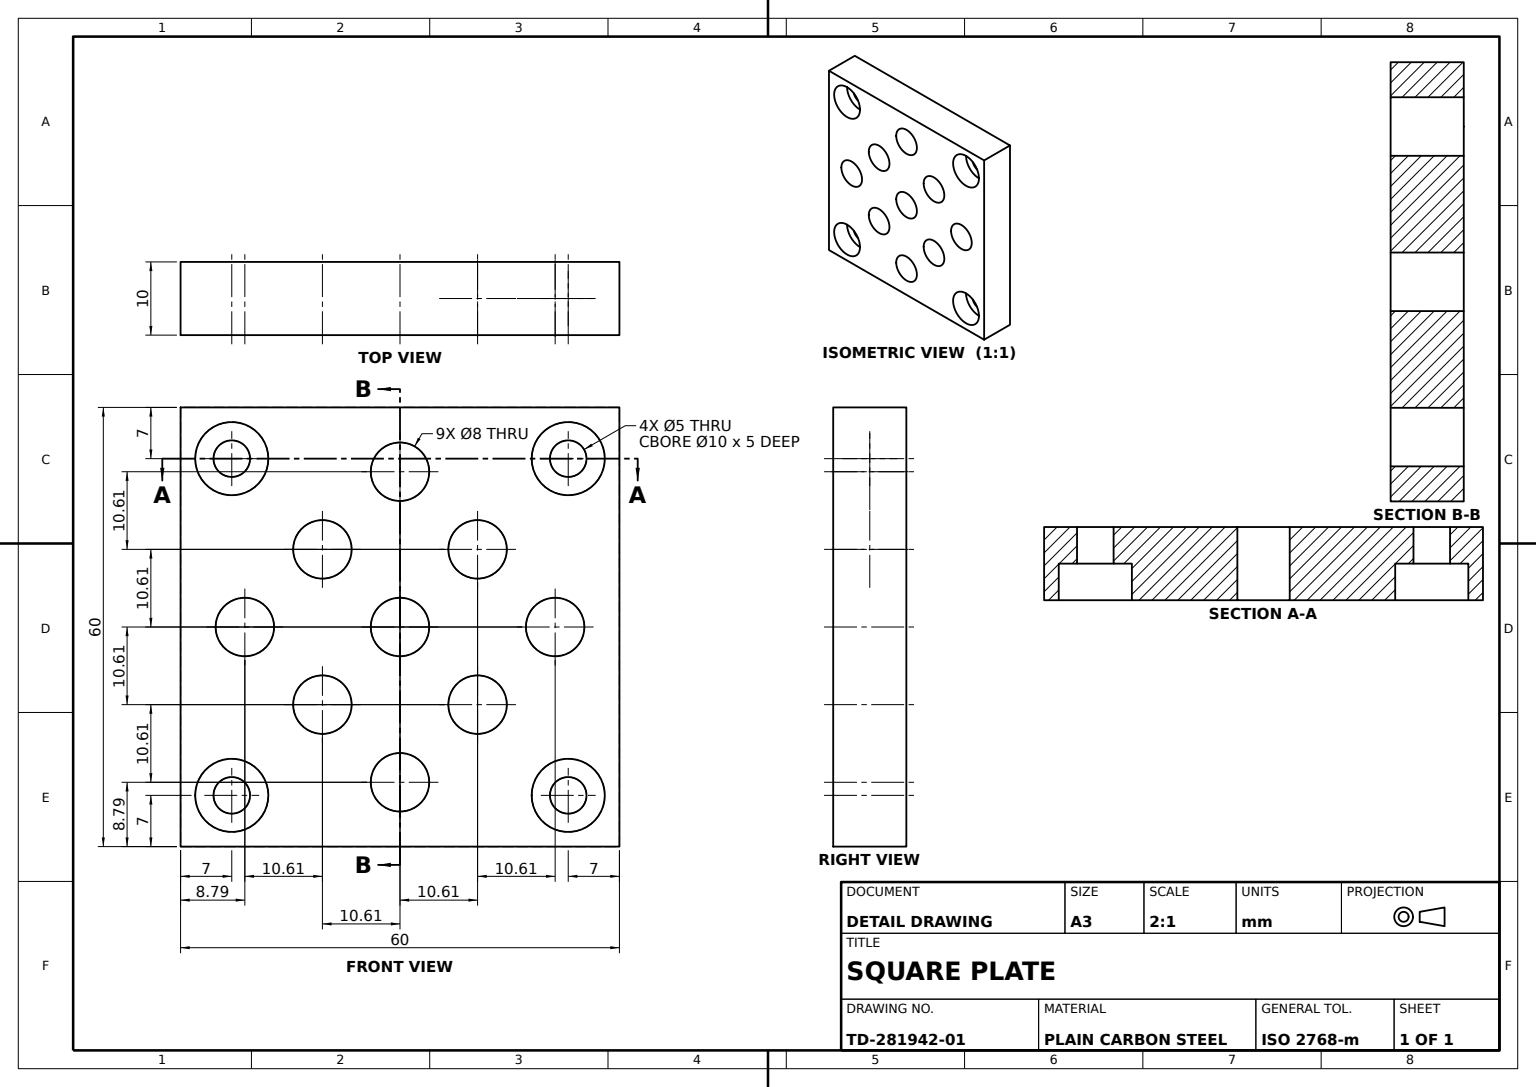
from build123d import *

# Parameters (mm, degrees)
PLATE_PROFILE_60X60_W           = 60
PLATE_PROFILE_60X60_H           = 60
BASE_PLATE_60X60X10_DEPTH       = 10
COUNTERBORE_PROFILE_4X_10_R     = 5
CORNER_COUNTERBORES_4X_10_DEPTH = 5
CORNER_HOLE_PROFILE_4X_5_R      = 2.5
CORNER_HOLES_4X_5_DEPTH         = 5
INNER_THROUGH_HOLES_12X_DEPTH   = 10


with BuildPart() as part:
    # Plate Profile 60x60 → Base Plate 60x60x10 (new body)
    with BuildSketch(Plane.XY):
        with Locations((30, 30)):
            Rectangle(PLATE_PROFILE_60X60_W, PLATE_PROFILE_60X60_H)
    extrude(amount=BASE_PLATE_60X60X10_DEPTH)

    # Counterbore Profile 4xØ10 → Corner Counterbores 4xØ10 (cut)
    with BuildSketch(Plane.XY.offset(10)):
        with Locations((7, 53)):
            Circle(COUNTERBORE_PROFILE_4X_10_R)
        with Locations((53, 53)):
            Circle(COUNTERBORE_PROFILE_4X_10_R)
        with Locations((7, 7)):
            Circle(COUNTERBORE_PROFILE_4X_10_R)
        with Locations((53, 7)):
            Circle(COUNTERBORE_PROFILE_4X_10_R)
    extrude(amount=-CORNER_COUNTERBORES_4X_10_DEPTH, mode=Mode.SUBTRACT)

    # Corner Hole Profile 4xØ5 → Corner Holes 4xØ5 (cut)
    with BuildSketch(Plane.XY.offset(5)):
        with Locations((7, 53)):
            Circle(CORNER_HOLE_PROFILE_4X_5_R)
        with Locations((53, 53)):
            Circle(CORNER_HOLE_PROFILE_4X_5_R)
        with Locations((7, 7)):
            Circle(CORNER_HOLE_PROFILE_4X_5_R)
        with Locations((53, 7)):
            Circle(CORNER_HOLE_PROFILE_4X_5_R)
    extrude(amount=-CORNER_HOLES_4X_5_DEPTH, mode=Mode.SUBTRACT)

    # Inner Hole Grid Profile → Inner Through Holes 12x (cut)
    with BuildSketch(Plane.XY.offset(10)):
        with BuildLine():
            Line((22.221825407, 37.778174593), (19.393398282, 40.606601718))
            Line((19.393398282, 40.606601718), (16.564971157, 43.435028843))
            ThreePointArc((16.564971157, 43.435028843), (16.564971157, 37.778174593), (22.221825407, 37.778174593))
        make_face()
        with BuildLine():
            ThreePointArc((22.221825407, 37.778174593), (23.088916412, 39.075867988), (23.393398282, 40.606601718))
            Line((23.393398282, 40.606601718), (19.393398282, 40.606601718))
            Line((19.393398282, 40.606601718), (22.221825407, 37.778174593))
        make_face()
        with BuildLine():
            Line((19.393398282, 40.606601718), (23.393398282, 40.606601718))
            ThreePointArc((23.393398282, 40.606601718), (20.924132012, 44.302119848), (16.564971157, 43.435028843))
            Line((16.564971157, 43.435028843), (19.393398282, 40.606601718))
        make_face()
        with BuildLine():
            Line((30, 51.213203436), (30, 55.213203436))
            ThreePointArc((30, 55.213203436), (26, 51.213203436), (30, 47.213203436))
            Line((30, 47.213203436), (30, 51.213203436))
        make_face()
        with BuildLine():
            ThreePointArc((34, 51.213203436), (32.828427125, 54.04163056), (30, 55.213203436))
            Line((30, 55.213203436), (30, 51.213203436))
            Line((30, 51.213203436), (32.828427125, 48.384776311))
            ThreePointArc((32.828427125, 48.384776311), (33.69551813, 49.682469706), (34, 51.213203436))
        make_face()
        with BuildLine():
            Line((32.828427125, 48.384776311), (30, 51.213203436))
            Line((30, 51.213203436), (30, 47.213203436))
            ThreePointArc((30, 47.213203436), (31.530733729, 47.517685306), (32.828427125, 48.384776311))
        make_face()
        with BuildLine():
            Line((40.606601718, 40.606601718), (37.778174593, 43.435028843))
            ThreePointArc((37.778174593, 43.435028843), (36.911083588, 42.137335447), (36.606601718, 40.606601718))
            Line((36.606601718, 40.606601718), (40.606601718, 40.606601718))
        make_face()
        with BuildLine():
            ThreePointArc((43.435028843, 43.435028843), (40.606601718, 44.606601718), (37.778174593, 43.435028843))
            Line((37.778174593, 43.435028843), (40.606601718, 40.606601718))
            Line((40.606601718, 40.606601718), (43.435028843, 43.435028843))
        make_face()
        with BuildLine():
            Line((43.435028843, 37.778174593), (40.606601718, 40.606601718))
            Line((40.606601718, 40.606601718), (37.778174593, 37.778174593))
            ThreePointArc((37.778174593, 37.778174593), (40.606601718, 36.606601718), (43.435028843, 37.778174593))
        make_face()
        with BuildLine():
            Line((43.435028843, 43.435028843), (40.606601718, 40.606601718))
            Line((40.606601718, 40.606601718), (43.435028843, 37.778174593))
            ThreePointArc((43.435028843, 37.778174593), (44.302119848, 39.075867988), (44.606601718, 40.606601718))
            ThreePointArc((44.606601718, 40.606601718), (44.302119848, 42.137335447), (43.435028843, 43.435028843))
        make_face()
        with BuildLine():
            Line((40.606601718, 40.606601718), (36.606601718, 40.606601718))
            ThreePointArc((36.606601718, 40.606601718), (36.911083588, 39.075867988), (37.778174593, 37.778174593))
            Line((37.778174593, 37.778174593), (40.606601718, 40.606601718))
        make_face()
        with BuildLine():
            ThreePointArc((55.213203436, 30), (52.743937165, 33.69551813), (48.384776311, 32.828427125))
            Line((48.384776311, 32.828427125), (51.213203436, 30))
            Line((51.213203436, 30), (55.213203436, 30))
        make_face()
        with BuildLine():
            Line((51.213203436, 30), (48.384776311, 32.828427125))
            ThreePointArc((48.384776311, 32.828427125), (47.517685306, 31.530733729), (47.213203436, 30))
            Line((47.213203436, 30), (51.213203436, 30))
        make_face()
        with BuildLine():
            Line((51.213203436, 30), (47.213203436, 30))
            ThreePointArc((47.213203436, 30), (51.213203436, 26), (55.213203436, 30))
            Line((55.213203436, 30), (51.213203436, 30))
        make_face()
        with BuildLine():
            Line((40.606601718, 19.393398282), (37.778174593, 22.221825407))
            ThreePointArc((37.778174593, 22.221825407), (36.911083588, 20.924132012), (36.606601718, 19.393398282))
            Line((36.606601718, 19.393398282), (40.606601718, 19.393398282))
        make_face()
        with BuildLine():
            Line((40.606601718, 19.393398282), (36.606601718, 19.393398282))
            ThreePointArc((36.606601718, 19.393398282), (39.075867988, 15.697880152), (43.435028843, 16.564971157))
            Line((43.435028843, 16.564971157), (40.606601718, 19.393398282))
        make_face()
        with BuildLine():
            ThreePointArc((44.606601718, 19.393398282), (42.137335447, 23.088916412), (37.778174593, 22.221825407))
            Line((37.778174593, 22.221825407), (40.606601718, 19.393398282))
            Line((40.606601718, 19.393398282), (43.435028843, 16.564971157))
            ThreePointArc((43.435028843, 16.564971157), (44.302119848, 17.862664553), (44.606601718, 19.393398282))
        make_face()
        with BuildLine():
            Line((22.221825407, 16.564971157), (19.393398282, 19.393398282))
            Line((19.393398282, 19.393398282), (16.564971157, 22.221825407))
            ThreePointArc((16.564971157, 22.221825407), (16.564971157, 16.564971157), (22.221825407, 16.564971157))
        make_face()
        with BuildLine():
            ThreePointArc((11.615223689, 27.171572875), (12.482314694, 28.469266271), (12.786796564, 30))
            Line((12.786796564, 30), (8.786796564, 30))
            Line((8.786796564, 30), (11.615223689, 27.171572875))
        make_face()
        with BuildLine():
            Line((11.615223689, 27.171572875), (8.786796564, 30))
            Line((8.786796564, 30), (4.786796564, 30))
            ThreePointArc((4.786796564, 30), (7.256062835, 26.30448187), (11.615223689, 27.171572875))
        make_face()
        with BuildLine():
            Line((8.786796564, 30), (12.786796564, 30))
            ThreePointArc((12.786796564, 30), (8.786796564, 34), (4.786796564, 30))
            Line((4.786796564, 30), (8.786796564, 30))
        make_face()
        with BuildLine():
            ThreePointArc((34, 8.786796564), (32.828427125, 11.615223689), (30, 12.786796564))
            Line((30, 12.786796564), (30, 8.786796564))
            Line((30, 8.786796564), (30, 4.786796564))
            ThreePointArc((30, 4.786796564), (32.828427125, 5.95836944), (34, 8.786796564))
        make_face()
        with BuildLine():
            Line((30, 8.786796564), (30, 12.786796564))
            ThreePointArc((30, 12.786796564), (28.469266271, 12.482314694), (27.171572875, 11.615223689))
            Line((27.171572875, 11.615223689), (30, 8.786796564))
        make_face()
        with BuildLine():
            Line((30, 4.786796564), (30, 8.786796564))
            Line((30, 8.786796564), (27.171572875, 11.615223689))
            ThreePointArc((27.171572875, 11.615223689), (26.30448187, 7.256062835), (30, 4.786796564))
        make_face()
        with BuildLine():
            Line((19.393398282, 19.393398282), (22.221825407, 22.221825407))
            ThreePointArc((22.221825407, 22.221825407), (19.393398282, 23.393398282), (16.564971157, 22.221825407))
            Line((16.564971157, 22.221825407), (19.393398282, 19.393398282))
        make_face()
        with BuildLine():
            ThreePointArc((23.393398282, 19.393398282), (23.088916412, 20.924132012), (22.221825407, 22.221825407))
            Line((22.221825407, 22.221825407), (19.393398282, 19.393398282))
            Line((19.393398282, 19.393398282), (23.393398282, 19.393398282))
        make_face()
        with BuildLine():
            ThreePointArc((22.221825407, 16.564971157), (23.088916412, 17.862664553), (23.393398282, 19.393398282))
            Line((23.393398282, 19.393398282), (19.393398282, 19.393398282))
            Line((19.393398282, 19.393398282), (22.221825407, 16.564971157))
        make_face()
        with BuildLine():
            Line((26, 30), (30, 30))
            Line((30, 30), (27.171572875, 32.828427125))
            ThreePointArc((27.171572875, 32.828427125), (26.30448187, 31.530733729), (26, 30))
        make_face()
        with BuildLine():
            Line((34, 30), (30, 30))
            Line((30, 30), (32.828427125, 27.171572875))
            ThreePointArc((32.828427125, 27.171572875), (33.69551813, 28.469266271), (34, 30))
        make_face()
        with BuildLine():
            Line((32.828427125, 32.828427125), (30, 30))
            Line((30, 30), (34, 30))
            ThreePointArc((34, 30), (33.69551813, 31.530733729), (32.828427125, 32.828427125))
        make_face()
        with BuildLine():
            ThreePointArc((32.828427125, 32.828427125), (31.530733729, 33.69551813), (30, 34))
            Line((30, 34), (30, 30))
            Line((30, 30), (32.828427125, 32.828427125))
        make_face()
        with BuildLine():
            Line((30, 30), (30, 34))
            ThreePointArc((30, 34), (28.469266271, 33.69551813), (27.171572875, 32.828427125))
            Line((27.171572875, 32.828427125), (30, 30))
        make_face()
        with BuildLine():
            Line((32.828427125, 27.171572875), (30, 30))
            Line((30, 30), (30, 26))
            ThreePointArc((30, 26), (31.530733729, 26.30448187), (32.828427125, 27.171572875))
        make_face()
        with BuildLine():
            Line((27.171572875, 27.171572875), (30, 30))
            Line((30, 30), (26, 30))
            ThreePointArc((26, 30), (26.30448187, 28.469266271), (27.171572875, 27.171572875))
        make_face()
        with BuildLine():
            Line((30, 26), (30, 30))
            Line((30, 30), (27.171572875, 27.171572875))
            ThreePointArc((27.171572875, 27.171572875), (28.469266271, 26.30448187), (30, 26))
        make_face()
    extrude(amount=-INNER_THROUGH_HOLES_12X_DEPTH, mode=Mode.SUBTRACT)


solid = part.part
